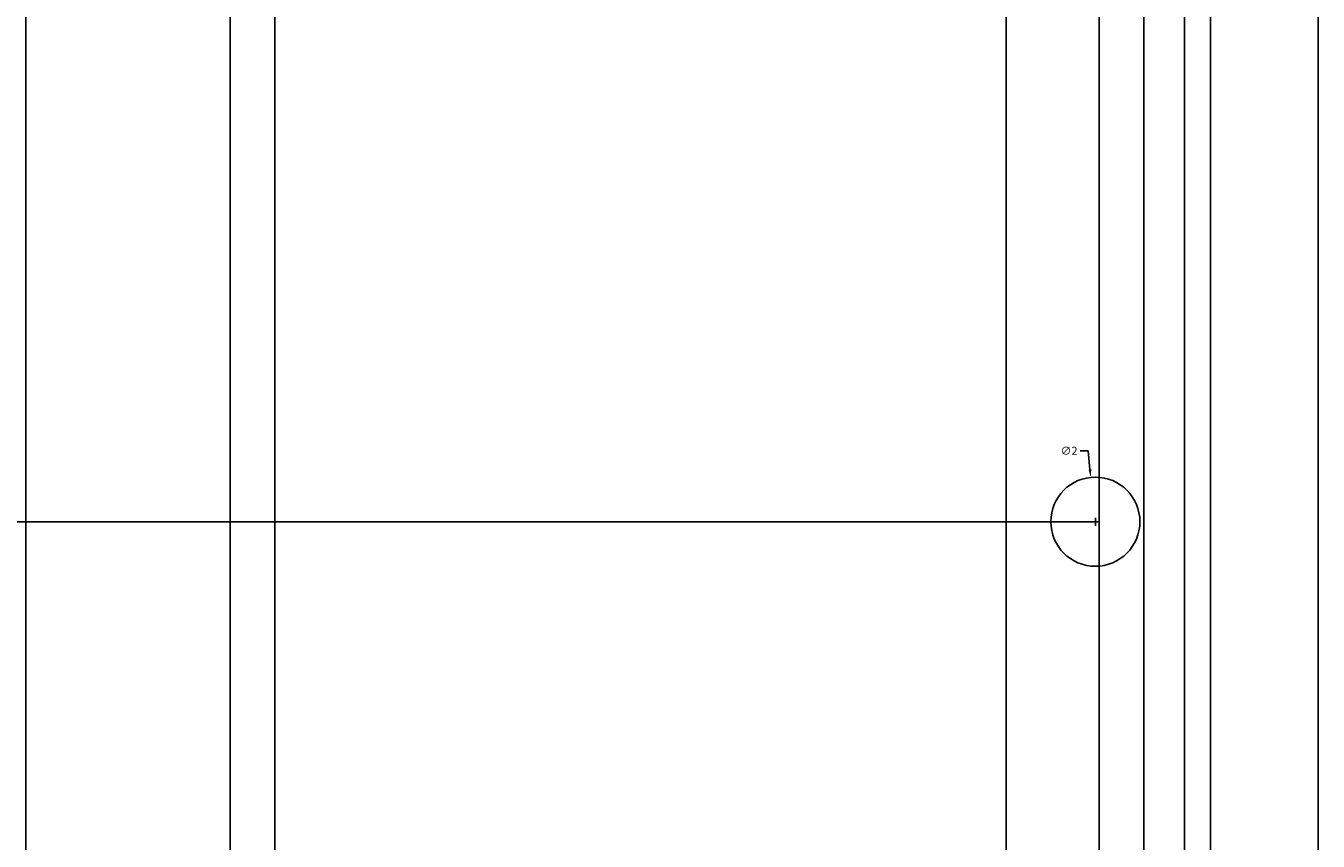
# Model space of a CAD drawing. Units: inches. Extents: x -6 to 289, y -8 to 323.
# Tile 23 of 107: x 142 to 171, y 69 to 87. Entities that reach past the tile are written whole.
import ezdxf

# ---------------------------------------------------------------- set-up
doc = ezdxf.new("R2010")
doc.units = ezdxf.units.IN
doc.header["$MEASUREMENT"] = 0
doc.layers.add('A-ANNO-DIMS', color=2, linetype='Continuous', lineweight=18)
doc.layers.add('A-DOOR', color=3, linetype='Continuous', lineweight=25)
doc.styles.get("Standard").update_dxf_attribs({"font": 'arial.ttf'})
doc.dimstyles.get("Standard").update_dxf_attribs({"dimtxt": 0.18, "dimasz": 0.18, "dimexe": 0.18, "dimexo": 0.0625, "dimgap": 0.09, "dimtad": 0, "dimtih": 1, "dimtoh": 1, "dimdec": 4, "dimzin": 0, "dimdsep": 46, "dimtxsty": 'Standard', "dimcen": 0.09, "dimadec": 0, "dimazin": 0, "dimtfac": 1, "dimtdec": 4, "dimtofl": 0, "dimtmove": 0, "dimatfit": 3, "dimfxl": 1, "dimtolj": 1, "dimtzin": 0, "dimarcsym": 0})

# ---------------------------------------------------------------- blocks, each defined once
blk = doc.blocks.new('*D30')
at = {"layer": 'A-ANNO-DIMS', "color": 0, "lineweight": -2, "transparency": 16777216}
for p, q in [((129.383, 181.092), (129.383, -8.391)), ((146.883, 181.092), (146.883, -8.391)), ((129.563, -8.211), (137.817, -8.211)), ((146.703, -8.211), (138.449, -8.211))]:
    blk.add_line(p, q, dxfattribs=at)
at = {"layer": 'A-ANNO-DIMS', "color": 0, "transparency": 16777216}
for points in [[(129.563, -8.181), (129.563, -8.241), (129.383, -8.211)], [(146.703, -8.181), (146.703, -8.241), (146.883, -8.211)]]:
    blk.add_solid(points, dxfattribs=at)
at = {"layer": 'Defpoints', "color": 0, "transparency": 16777216}
for p in [(129.383, 181.154), (146.883, 181.154), (146.883, -8.211)]:
    blk.add_point(p, dxfattribs=at)
at = {"layer": 'A-ANNO-DIMS', "color": 0, "transparency": 16777216, "insert": (138.133, -8.211), "char_height": 0.18, "attachment_point": 5}
blk.add_mtext('\\A1;17.5', dxfattribs=at)
blk = doc.blocks.new('*D31')
at = {"layer": 'A-ANNO-DIMS', "color": 0, "lineweight": -2, "transparency": 16777216}
for p, q in [((146.883, 181.092), (146.883, -8.391)), ((147.883, 181.092), (147.883, -8.391)), ((147.063, -8.211), (147.26, -8.211)), ((147.703, -8.211), (147.507, -8.211))]:
    blk.add_line(p, q, dxfattribs=at)
at = {"layer": 'A-ANNO-DIMS', "color": 0, "transparency": 16777216}
for points in [[(147.063, -8.181), (147.063, -8.241), (146.883, -8.211)], [(147.703, -8.181), (147.703, -8.241), (147.883, -8.211)]]:
    blk.add_solid(points, dxfattribs=at)
at = {"layer": 'Defpoints', "color": 0, "transparency": 16777216}
for p in [(146.883, 181.154), (147.883, 181.154), (147.883, -8.211)]:
    blk.add_point(p, dxfattribs=at)
at = {"layer": 'A-ANNO-DIMS', "color": 0, "transparency": 16777216, "insert": (147.383, -8.211), "char_height": 0.18, "attachment_point": 5}
blk.add_mtext('\\A1;1', dxfattribs=at)
blk = doc.blocks.new('*D32')
at = {"layer": 'A-ANNO-DIMS', "color": 0, "lineweight": -2, "transparency": 16777216}
for p, q in [((147.883, 181.092), (147.883, -8.391)), ((166.383, 181.092), (166.383, -8.391)), ((148.063, -8.211), (156.817, -8.211)), ((166.203, -8.211), (157.449, -8.211))]:
    blk.add_line(p, q, dxfattribs=at)
at = {"layer": 'A-ANNO-DIMS', "color": 0, "transparency": 16777216}
for points in [[(148.063, -8.181), (148.063, -8.241), (147.883, -8.211)], [(166.203, -8.181), (166.203, -8.241), (166.383, -8.211)]]:
    blk.add_solid(points, dxfattribs=at)
at = {"layer": 'Defpoints', "color": 0, "transparency": 16777216}
for p in [(147.883, 181.154), (166.383, 181.154), (166.383, -8.211)]:
    blk.add_point(p, dxfattribs=at)
at = {"layer": 'A-ANNO-DIMS', "color": 0, "transparency": 16777216, "insert": (157.133, -8.211), "char_height": 0.18, "attachment_point": 5}
blk.add_mtext('\\A1;18.5', dxfattribs=at)
blk = doc.blocks.new('*D33')
at = {"layer": 'A-ANNO-DIMS', "color": 0, "lineweight": -2, "transparency": 16777216}
for p, q in [((166.383, 181.092), (166.383, -8.391)), ((167.383, 180.092), (167.383, -8.391)), ((166.563, -8.211), (166.76, -8.211)), ((167.203, -8.211), (167.007, -8.211))]:
    blk.add_line(p, q, dxfattribs=at)
at = {"layer": 'A-ANNO-DIMS', "color": 0, "transparency": 16777216}
for points in [[(166.563, -8.181), (166.563, -8.241), (166.383, -8.211)], [(167.203, -8.181), (167.203, -8.241), (167.383, -8.211)]]:
    blk.add_solid(points, dxfattribs=at)
at = {"layer": 'Defpoints', "color": 0, "transparency": 16777216}
for p in [(166.383, 181.154), (167.383, 180.154), (167.383, -8.211)]:
    blk.add_point(p, dxfattribs=at)
at = {"layer": 'A-ANNO-DIMS', "color": 0, "transparency": 16777216, "insert": (166.883, -8.211), "char_height": 0.18, "attachment_point": 5}
blk.add_mtext('\\A1;1', dxfattribs=at)
blk = doc.blocks.new('*D34')
at = {"layer": 'A-ANNO-DIMS', "color": 0, "lineweight": -2, "transparency": 16777216}
for p, q in [((167.383, 180.092), (167.383, -8.391)), ((168.883, 178.592), (168.883, -8.391)), ((167.563, -8.211), (167.887, -8.211)), ((168.703, -8.211), (168.38, -8.211))]:
    blk.add_line(p, q, dxfattribs=at)
at = {"layer": 'A-ANNO-DIMS', "color": 0, "transparency": 16777216}
for points in [[(167.563, -8.181), (167.563, -8.241), (167.383, -8.211)], [(168.703, -8.181), (168.703, -8.241), (168.883, -8.211)]]:
    blk.add_solid(points, dxfattribs=at)
at = {"layer": 'Defpoints', "color": 0, "transparency": 16777216}
for p in [(167.383, 180.154), (168.883, 178.654), (168.883, -8.211)]:
    blk.add_point(p, dxfattribs=at)
at = {"layer": 'A-ANNO-DIMS', "color": 0, "transparency": 16777216, "insert": (168.133, -8.211), "char_height": 0.18, "attachment_point": 5}
blk.add_mtext('\\A1;1.5', dxfattribs=at)
blk = doc.blocks.new('*D76')
at = {"layer": 'A-ANNO-DIMS', "color": 0, "lineweight": -2, "transparency": 16777216}
for p, q in [((142.296, 51.148), (142.296, 322.969)), ((142.476, 322.789), (153.076, 322.789)), ((164.116, 322.789), (153.516, 322.789)), ((164.296, 51.148), (164.296, 322.969))]:
    blk.add_line(p, q, dxfattribs=at)
at = {"layer": 'A-ANNO-DIMS', "color": 0, "transparency": 16777216}
for points in [[(142.476, 322.819), (142.476, 322.759), (142.296, 322.789)], [(164.116, 322.819), (164.116, 322.759), (164.296, 322.789)]]:
    blk.add_solid(points, dxfattribs=at)
at = {"layer": 'Defpoints', "color": 0, "transparency": 16777216}
for p in [(164.296, 322.789), (142.296, 51.085), (164.296, 51.085)]:
    blk.add_point(p, dxfattribs=at)
at = {"layer": 'A-ANNO-DIMS', "color": 0, "transparency": 16777216, "insert": (153.296, 322.789), "char_height": 0.18, "attachment_point": 5}
blk.add_mtext('\\A1;22', dxfattribs=at)
blk = doc.blocks.new('*D77')
at = {"layer": 'A-ANNO-DIMS', "color": 0, "lineweight": -2, "transparency": 16777216}
for p, q in [((164.296, 51.148), (164.296, 322.969)), ((164.476, 322.789), (166.144, 322.789)), ((168.116, 322.789), (166.448, 322.789)), ((168.296, 51.148), (168.296, 322.969))]:
    blk.add_line(p, q, dxfattribs=at)
at = {"layer": 'A-ANNO-DIMS', "color": 0, "transparency": 16777216}
for points in [[(164.476, 322.819), (164.476, 322.759), (164.296, 322.789)], [(168.116, 322.819), (168.116, 322.759), (168.296, 322.789)]]:
    blk.add_solid(points, dxfattribs=at)
at = {"layer": 'Defpoints', "color": 0, "transparency": 16777216}
for p in [(168.296, 322.789), (164.296, 51.085), (168.296, 51.085)]:
    blk.add_point(p, dxfattribs=at)
at = {"layer": 'A-ANNO-DIMS', "color": 0, "transparency": 16777216, "insert": (166.296, 322.789), "char_height": 0.18, "attachment_point": 5}
blk.add_mtext('\\A1;4', dxfattribs=at)
blk = doc.blocks.new('*D78')
at = {"layer": 'A-ANNO-DIMS', "color": 0, "lineweight": -2, "transparency": 16777216}
for p, q in [((168.296, 51.148), (168.296, 322.969)), ((168.476, 322.789), (169.647, 322.789)), ((171.116, 322.789), (169.945, 322.789)), ((171.296, 51.148), (171.296, 322.969))]:
    blk.add_line(p, q, dxfattribs=at)
at = {"layer": 'A-ANNO-DIMS', "color": 0, "transparency": 16777216}
for points in [[(168.476, 322.819), (168.476, 322.759), (168.296, 322.789)], [(171.116, 322.819), (171.116, 322.759), (171.296, 322.789)]]:
    blk.add_solid(points, dxfattribs=at)
at = {"layer": 'Defpoints', "color": 0, "transparency": 16777216}
for p in [(171.296, 322.789), (168.296, 51.085), (171.296, 51.085)]:
    blk.add_point(p, dxfattribs=at)
at = {"layer": 'A-ANNO-DIMS', "color": 0, "transparency": 16777216, "insert": (169.796, 322.789), "char_height": 0.18, "attachment_point": 5}
blk.add_mtext('\\A1;3', dxfattribs=at)
blk = doc.blocks.new('*D86')
at = {"layer": 'A-ANNO-DIMS', "color": 0, "lineweight": -2, "transparency": 16777216}
for p, q in [((166.233, 75.971), (-5.737, 75.971)), ((-5.557, 75.791), (-5.557, 63.71)), ((-5.557, 51.265), (-5.557, 63.346)), ((120.945, 51.085), (-5.737, 51.085))]:
    blk.add_line(p, q, dxfattribs=at)
at = {"layer": 'A-ANNO-DIMS', "color": 0, "transparency": 16777216}
for points in [[(-5.587, 75.791), (-5.527, 75.791), (-5.557, 75.971)], [(-5.587, 51.265), (-5.527, 51.265), (-5.557, 51.085)]]:
    blk.add_solid(points, dxfattribs=at)
at = {"layer": 'Defpoints', "color": 0, "transparency": 16777216}
for p in [(-5.557, 75.971), (166.296, 75.971), (121.008, 51.085)]:
    blk.add_point(p, dxfattribs=at)
at = {"layer": 'A-ANNO-DIMS', "color": 0, "transparency": 16777216, "insert": (-5.557, 63.528), "char_height": 0.18, "attachment_point": 5}
blk.add_mtext('\\A1;24.886', dxfattribs=at)
blk = doc.blocks.new('*D87')
at = {"layer": 'A-ANNO-DIMS', "color": 0, "lineweight": -2, "transparency": 16777216}
for p, q in [((142.233, 108.948), (-5.737, 108.948)), ((-5.557, 108.768), (-5.557, 92.641)), ((-5.557, 76.151), (-5.557, 92.277)), ((166.233, 75.971), (-5.737, 75.971))]:
    blk.add_line(p, q, dxfattribs=at)
at = {"layer": 'A-ANNO-DIMS', "color": 0, "transparency": 16777216}
for points in [[(-5.587, 108.768), (-5.527, 108.768), (-5.557, 108.948)], [(-5.587, 76.151), (-5.527, 76.151), (-5.557, 75.971)]]:
    blk.add_solid(points, dxfattribs=at)
at = {"layer": 'Defpoints', "color": 0, "transparency": 16777216}
for p in [(-5.557, 108.948), (142.296, 108.948), (166.296, 75.971)]:
    blk.add_point(p, dxfattribs=at)
at = {"layer": 'A-ANNO-DIMS', "color": 0, "transparency": 16777216, "insert": (-5.557, 92.459), "char_height": 0.18, "attachment_point": 5}
blk.add_mtext('\\A1;32.98', dxfattribs=at)
blk = doc.blocks.new('*D119')
at = {"layer": 'A-ANNO-DIMS', "color": 0, "lineweight": -2, "transparency": 16777216}
for p, q in [((165.952, 77.562), (166.132, 77.562)), ((166.132, 77.562), (166.175, 77.144)), ((166.296, 75.881), (166.296, 76.061)), ((166.206, 75.971), (166.386, 75.971))]:
    blk.add_line(p, q, dxfattribs=at)
at = {"layer": 'A-ANNO-DIMS', "color": 0, "transparency": 16777216}
blk.add_solid([(166.205, 77.147), (166.145, 77.141), (166.193, 76.965)], dxfattribs=at)
at = {"layer": 'Defpoints', "color": 0, "transparency": 16777216}
for p in [(166.193, 76.965), (166.399, 74.976)]:
    blk.add_point(p, dxfattribs=at)
at = {"layer": 'A-ANNO-DIMS', "color": 0, "transparency": 16777216, "insert": (165.706, 77.562), "char_height": 0.18, "attachment_point": 5}
blk.add_mtext('\\A1;∅2', dxfattribs=at)

msp = doc.modelspace()

# ---------------------------------------------------------------- linework, layer by layer
at = {"layer": 'A-DOOR'}
for points in [[(135.296, 51.0851), (135.296, 117.9706), (171.296, 117.9706), (171.296, 51.0851)], [(138.296, 51.0851), (138.296, 114.9477), (168.296, 114.9477), (168.296, 51.0851)], [(164.296, 51.0851), (164.296, 108.9477), (142.296, 108.9477), (142.296, 51.0851)]]:
    msp.add_lwpolyline(points, dxfattribs=at)
msp.add_circle((166.296, 75.9706), 1, dxfattribs=at)

# ---------------------------------------------------------------- dimensions: what is measured, and where the dimension line sits
at = {"layer": 'A-ANNO-DIMS'}
for base, p1, p2, override, picture, middle in [((164.296, 322.7888), (142.296, 51.0851), (164.296, 51.0851), {"dimdec": 0, "dimlfac": 1, "dimrnd": 0, "dimzin": 0, "dimdsep": 46, "dimlunit": 2}, '*D76', (153.296, 322.7888)), ((168.296, 322.7888), (164.296, 51.0851), (168.296, 51.0851), {"dimdec": 0, "dimlfac": 1, "dimrnd": 0, "dimzin": 0, "dimdsep": 46, "dimlunit": 2}, '*D77', (166.296, 322.7888)), ((171.296, 322.7888), (168.296, 51.0851), (171.296, 51.0851), {"dimdec": 0, "dimlfac": 1, "dimrnd": 0, "dimzin": 0, "dimdsep": 46, "dimlunit": 2}, '*D78', (169.796, 322.7888)), ((146.8835, -8.2112), (129.3835, 181.154), (146.8835, 181.154), {"dimdec": 1, "dimlfac": 1, "dimrnd": 0, "dimzin": 0, "dimdsep": 46, "dimlunit": 2}, '*D30', (138.1335, -8.2112)), ((147.8835, -8.2112), (146.8835, 181.154), (147.8835, 181.154), {"dimdec": 0, "dimlfac": 1, "dimrnd": 0, "dimzin": 0, "dimdsep": 46, "dimlunit": 2}, '*D31', (147.3835, -8.2112)), ((166.3835, -8.2112), (147.8835, 181.154), (166.3835, 181.154), {"dimdec": 1, "dimlfac": 1, "dimrnd": 0, "dimzin": 0, "dimdsep": 46, "dimlunit": 2}, '*D32', (157.1335, -8.2112)), ((167.3835, -8.2112), (166.3835, 181.154), (167.3835, 180.154), {"dimdec": 0, "dimlfac": 1, "dimrnd": 0, "dimzin": 0, "dimdsep": 46, "dimlunit": 2}, '*D33', (166.8835, -8.2112)), ((168.8835, -8.2112), (167.3835, 180.154), (168.8835, 178.654), {"dimdec": 1, "dimlfac": 1, "dimrnd": 0, "dimzin": 0, "dimdsep": 46, "dimlunit": 2}, '*D34', (168.1335, -8.2112))]:
    dim = msp.add_linear_dim(base=base, p1=p1, p2=p2, dimstyle='Standard', override=override, dxfattribs=at)
    dim.commit()
    dim.dimension.update_dxf_attribs({"geometry": picture, "text_midpoint": middle})
for base, p1, p2, override, picture, middle in [((-5.557, 108.9477), (166.296, 75.9706), (142.296, 108.9477), {"dimdec": 2, "dimlfac": 1, "dimrnd": 0, "dimzin": 0, "dimdsep": 46, "dimlunit": 2}, '*D87', (-5.557, 92.4592)), ((-5.557, 75.97064), (121.00798, 51.08513), (166.29599, 75.97064), {"dimdec": 3, "dimlfac": 1, "dimrnd": 0, "dimzin": 0, "dimdsep": 46, "dimlunit": 2}, '*D86', (-5.557, 63.52788))]:
    dim = msp.add_linear_dim(base=base, p1=p1, p2=p2, angle=90, dimstyle='Standard', override=override, dxfattribs=at)
    dim.commit()
    dim.dimension.update_dxf_attribs({"geometry": picture, "text_midpoint": middle})
dim = msp.add_diameter_dim_2p(p1=(166.3987, 74.9759), p2=(166.1932, 76.9654), dimstyle='Standard', override={"dimdec": 0, "dimlfac": 1, "dimrnd": 0, "dimzin": 0, "dimdsep": 46, "dimlunit": 2}, dxfattribs=at)
dim.commit()
dim.dimension.update_dxf_attribs({"geometry": '*D119', "text_midpoint": (165.7056, 77.5622), "dimtype": 163})

doc.saveas('drawing.dxf')
